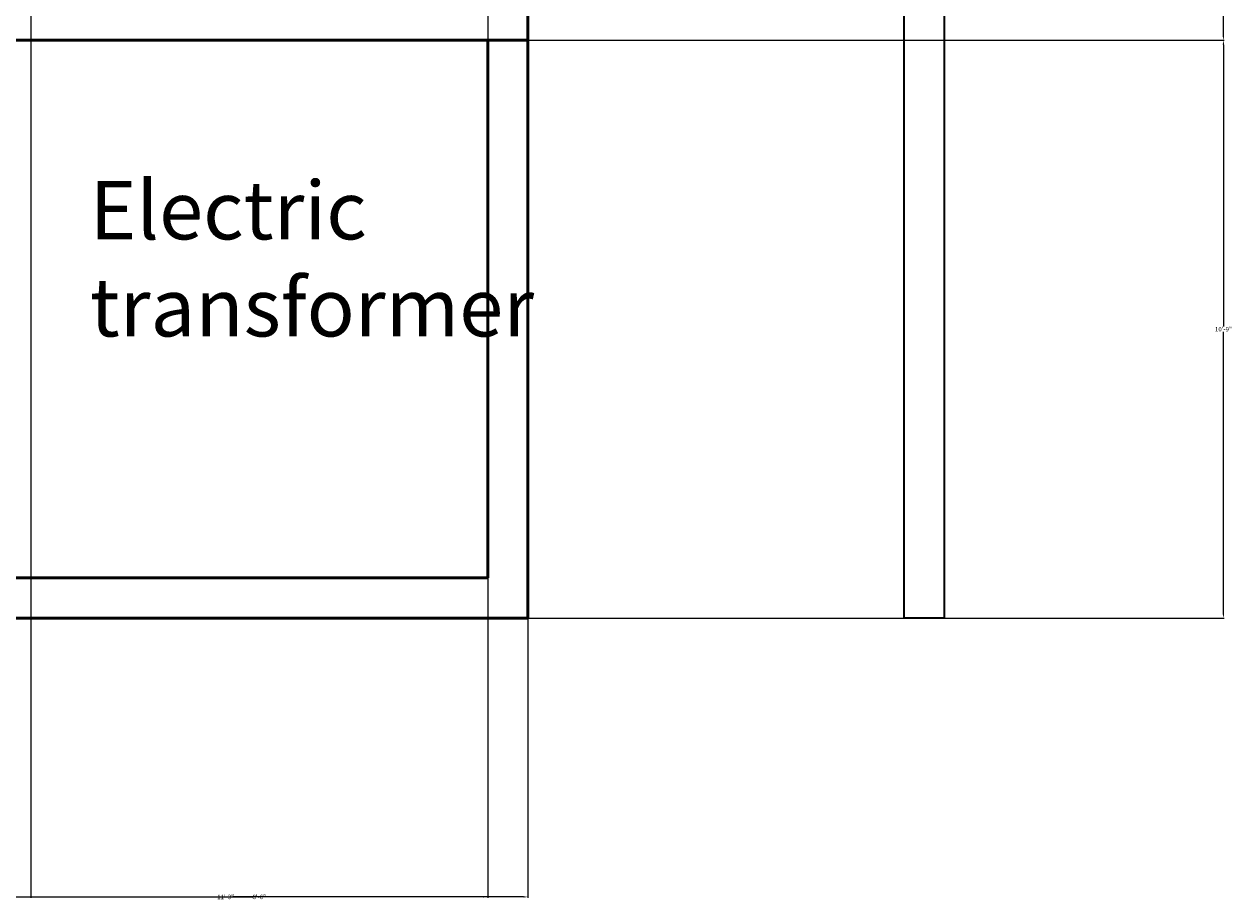
# Model space of a CAD drawing. Units: inches. Extents: x -364 to 705, y -52 to 1250.
# Tile 13 of 34: x 435 to 705, y -52 to 144. Entities that reach past the tile are written whole.
import ezdxf

# ---------------------------------------------------------------- set-up
doc = ezdxf.new("R2010")
doc.units = ezdxf.units.IN
doc.header["$MEASUREMENT"] = 0
for name, color, linetype, lineweight in [('A-ANNO-DIMS', 4, 'Continuous', 18), ('A-ANNO-TEXT', 3, 'Continuous', 18), ('A-WALL', 41, 'Continuous', 50), ('C-WALL', 41, 'Continuous', 35)]:
    doc.layers.add(name, color=color, linetype=linetype, lineweight=lineweight)
doc.styles.get("Standard").update_dxf_attribs({"font": 'arial.ttf'})
doc.dimstyles.get("Standard").update_dxf_attribs({"dimtxt": 1, "dimasz": 1, "dimexe": 0.18, "dimexo": 0.0625, "dimgap": 0.09, "dimtad": 0, "dimtih": 1, "dimtoh": 1, "dimdec": 0, "dimzin": 0, "dimdsep": 46, "dimlunit": 3, "dimtxsty": 'Standard', "dimcen": 0.09, "dimadec": 0, "dimazin": 0, "dimtfac": 1, "dimtdec": 0, "dimtofl": 0, "dimtmove": 0, "dimatfit": 3, "dimfxl": 1, "dimtolj": 1, "dimtzin": 0, "dimarcsym": 0})

# ---------------------------------------------------------------- blocks, each defined once
blk = doc.blocks.new('*D77')
at = {"layer": 'A-ANNO-DIMS', "color": 0, "lineweight": -2, "transparency": 16777216}
for p, q in [((538.64, 140.11), (703.01, 140.11)), ((702.83, 139.11), (702.83, 76.22)), ((702.83, 12.11), (702.83, 75.01)), ((547.64, 11.11), (703.01, 11.11))]:
    blk.add_line(p, q, dxfattribs=at)
at = {"layer": 'A-ANNO-DIMS', "color": 0, "transparency": 16777216}
for points in [[(702.66, 139.11), (703, 139.11), (702.83, 140.11)], [(702.66, 12.11), (703, 12.11), (702.83, 11.11)]]:
    blk.add_solid(points, dxfattribs=at)
at = {"layer": 'Defpoints', "color": 0, "transparency": 16777216}
for p in [(538.58, 140.11), (702.83, 140.11), (547.58, 11.11)]:
    blk.add_point(p, dxfattribs=at)
at = {"layer": 'A-ANNO-DIMS', "color": 0, "transparency": 16777216, "insert": (702.83, 75.61), "char_height": 1, "attachment_point": 5}
blk.add_mtext('\\A1;10\'-9"', dxfattribs=at)
blk = doc.blocks.new('*D78')
at = {"layer": 'A-ANNO-DIMS', "color": 0, "lineweight": -2, "transparency": 16777216}
for p, q in [((538.64, 303.11), (703.01, 303.11)), ((702.83, 302.11), (702.83, 222.22)), ((702.83, 141.11), (702.83, 221.01)), ((538.64, 140.11), (703.01, 140.11))]:
    blk.add_line(p, q, dxfattribs=at)
at = {"layer": 'A-ANNO-DIMS', "color": 0, "transparency": 16777216}
for points in [[(702.66, 302.11), (703, 302.11), (702.83, 303.11)], [(702.66, 141.11), (703, 141.11), (702.83, 140.11)]]:
    blk.add_solid(points, dxfattribs=at)
at = {"layer": 'Defpoints', "color": 0, "transparency": 16777216}
for p in [(538.58, 303.11), (702.83, 303.11), (538.58, 140.11)]:
    blk.add_point(p, dxfattribs=at)
at = {"layer": 'A-ANNO-DIMS', "color": 0, "transparency": 16777216, "insert": (702.83, 221.61), "char_height": 1, "attachment_point": 5}
blk.add_mtext('\\A1;13\'-7"', dxfattribs=at)
blk = doc.blocks.new('*D89')
at = {"layer": 'A-ANNO-DIMS', "color": 0, "lineweight": -2, "transparency": 16777216}
for p, q in [((412.58, 20.05), (412.58, -51.32)), ((547.58, 11.05), (547.58, -51.32)), ((413.58, -51.14), (478.32, -51.14)), ((546.58, -51.14), (481.84, -51.14))]:
    blk.add_line(p, q, dxfattribs=at)
at = {"layer": 'A-ANNO-DIMS', "color": 0, "transparency": 16777216}
for points in [[(413.58, -50.97), (413.58, -51.3), (412.58, -51.14)], [(546.58, -50.97), (546.58, -51.3), (547.58, -51.14)]]:
    blk.add_solid(points, dxfattribs=at)
at = {"layer": 'Defpoints', "color": 0, "transparency": 16777216}
for p in [(412.58, 20.11), (547.58, 11.11), (547.58, -51.14)]:
    blk.add_point(p, dxfattribs=at)
at = {"layer": 'A-ANNO-DIMS', "color": 0, "transparency": 16777216, "insert": (480.08, -51.14), "char_height": 1, "attachment_point": 5}
blk.add_mtext('\\A1;11\'-3"', dxfattribs=at)
blk = doc.blocks.new('*D100')
at = {"layer": 'A-ANNO-DIMS', "color": 0, "lineweight": -2, "transparency": 16777216}
for p, q in [((436.58, 417.05), (436.58, -51.32)), ((538.58, 417.05), (538.58, -51.32)), ((437.58, -51.14), (486.16, -51.14)), ((537.58, -51.14), (489, -51.14))]:
    blk.add_line(p, q, dxfattribs=at)
at = {"layer": 'A-ANNO-DIMS', "color": 0, "transparency": 16777216}
for points in [[(437.58, -50.97), (437.58, -51.3), (436.58, -51.14)], [(537.58, -50.97), (537.58, -51.3), (538.58, -51.14)]]:
    blk.add_solid(points, dxfattribs=at)
at = {"layer": 'Defpoints', "color": 0, "transparency": 16777216}
for p in [(436.58, 417.11), (538.58, 417.11), (538.58, -51.14)]:
    blk.add_point(p, dxfattribs=at)
at = {"layer": 'A-ANNO-DIMS', "color": 0, "transparency": 16777216, "insert": (487.58, -51.14), "char_height": 1, "attachment_point": 5}
blk.add_mtext('\\A1;8\'-6"', dxfattribs=at)

msp = doc.modelspace()

# ---------------------------------------------------------------- linework, layer by layer
at = {"layer": 'A-WALL'}
for p, q in [((547.58, 11.11), (547.58, 986.11)), ((547.58, 140.11), (412.58, 140.11)), ((538.58, 20.11), (538.58, 140.11)), ((538.58, 20.11), (346.58, 20.11)), ((547.58, 11.11), (346.58, 11.11))]:
    msp.add_line(p, q, dxfattribs=at)
at = {"layer": 'C-WALL'}
for p, q in [((640.58, 11.11), (640.58, 1079.11)), ((631.58, 11.11), (631.58, 1070.11)), ((640.58, 11.11), (631.58, 11.11))]:
    msp.add_line(p, q, dxfattribs=at)

# ---------------------------------------------------------------- texts
at = {"layer": 'A-ANNO-TEXT', "insert": (449.74, 108.66), "char_height": 13, "attachment_point": 1}
msp.add_mtext_dynamic_manual_height_columns('Electric transformer', width=44.5593, gutter_width=0.69, heights=[0], dxfattribs=at)

# ---------------------------------------------------------------- dimensions: what is measured, and where the dimension line sits
at = {"layer": 'A-ANNO-DIMS'}
for base, p1, p2, picture, middle in [((538.58, -51.14), (436.58, 417.11), (538.58, 417.11), '*D100', (487.58, -51.14)), ((547.58, -51.14), (412.58, 20.11), (547.58, 11.11), '*D89', (480.08, -51.14))]:
    dim = msp.add_linear_dim(base=base, p1=p1, p2=p2, dimstyle='Standard', override={"dimdec": 1, "dimlfac": 1, "dimrnd": 0, "dimzin": 1, "dimdsep": 46, "dimlunit": 4, "dimfrac": 2}, dxfattribs=at)
    dim.commit()
    dim.dimension.update_dxf_attribs({"geometry": picture, "text_midpoint": middle})
for base, p1, p2, picture, middle in [((702.83, 303.11), (538.58, 140.11), (538.58, 303.11), '*D78', (702.83, 221.61)), ((702.83, 140.11), (547.58, 11.11), (538.58, 140.11), '*D77', (702.83, 75.61))]:
    dim = msp.add_linear_dim(base=base, p1=p1, p2=p2, angle=90, dimstyle='Standard', override={"dimdec": 1, "dimlfac": 1, "dimrnd": 0, "dimzin": 1, "dimdsep": 46, "dimlunit": 4, "dimfrac": 2}, dxfattribs=at)
    dim.commit()
    dim.dimension.update_dxf_attribs({"geometry": picture, "text_midpoint": middle})

doc.saveas('drawing.dxf')
